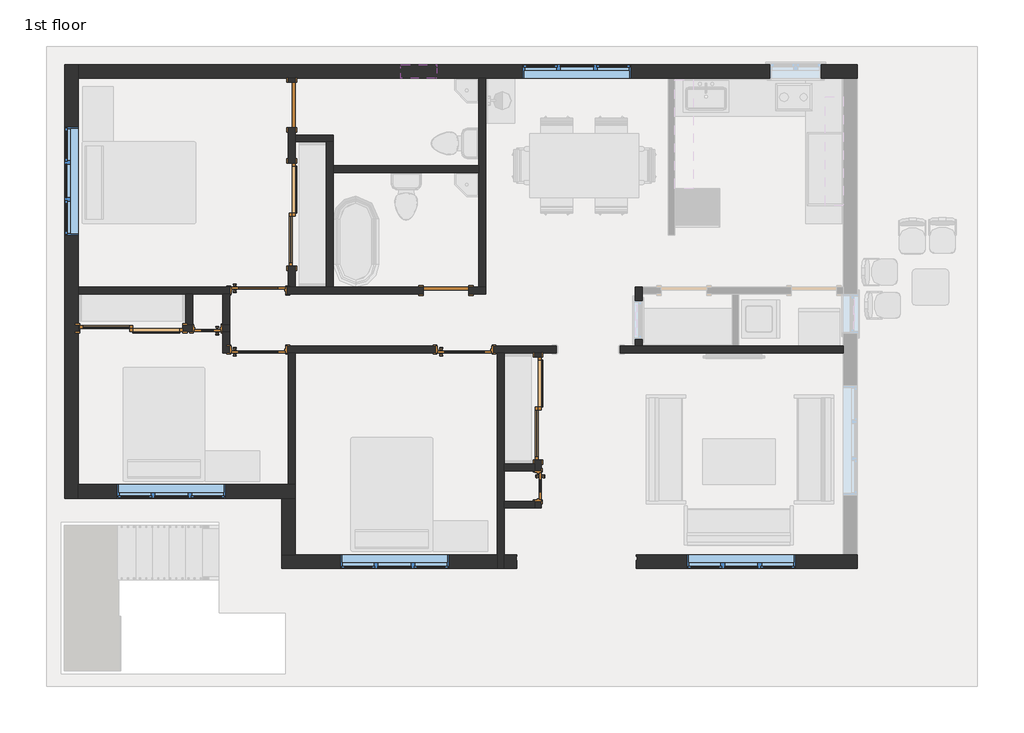
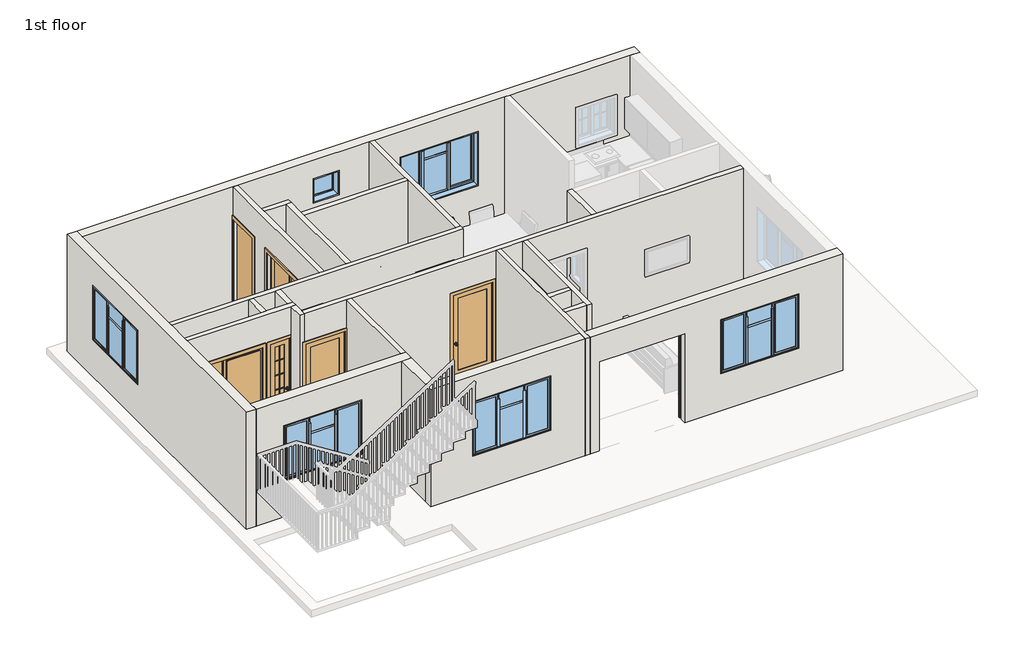
# One storey, part 1 of 4: 23 walls, 10 doors, 6 windows.
"""IFC4 building model written with IfcOpenShell, lengths in millimetres."""

from ifc_helpers import new_model, si_unit, frame, origin, place, context, project, spatial, polyline, outline, extrude, faceted_brep, transform, mapped, element, save
from components import door_505787c2, door_a3feeac7, door_3c6ab76a, door_ccf0cbd1, door_214872d5, door_78caadf7, window_80340324, window_7a1f68bc

model = new_model("IFC4")

# Units and contexts
model_context = context("Model", 3, world=origin())
ifc_project = project(units=[si_unit("LENGTHUNIT", "METRE", prefix="MILLI")], contexts=[model_context])

# Site, building, storey
site = spatial("IfcSite", under=ifc_project)
building = spatial("IfcBuilding", under=site)
storey = spatial("IfcBuildingStorey", under=building, Name="1st floor", Elevation=3810.0)

# Doors
placement = place(None, origin())
door_shape = door_505787c2(model_context)
element("IfcDoor", 1, ObjectType="Door-Double-Sliding : 68\" x 84\"", at=placement, inside=storey, context=model_context, shape_type="MappedRepresentation", body=[
    mapped(door_shape, transform((-1350.0263529, 910.5161978, 3810.0), x_axis=(0.0, -1.0, 0.0), y_axis=(1.0, 0.0, 0.0), z_axis=(0.0, 0.0, 1.0))),
])
element("IfcDoor", 2, ObjectType="Door-Double-Sliding : 68\" x 84\"", at=placement, inside=storey, context=model_context, shape_type="MappedRepresentation", body=[
    mapped(door_shape, transform((-8046.1013529, 2383.7161978, 3810.0), x_axis=(-1.0, 0.0, 0.0), y_axis=(0.0, -1.0, 0.0), z_axis=(0.0, 0.0, 1.0))),
])
element("IfcDoor", 3, ObjectType="Door-Double-Sliding : 68\" x 84\"", at=placement, inside=storey, context=model_context, shape_type="MappedRepresentation", body=[
    mapped(door_shape, transform((-5477.5263529, 4168.0661978, 3810.0), x_axis=(0.0, -1.0, 0.0), y_axis=(1.0, 0.0, 0.0), z_axis=(0.0, 0.0, 1.0))),
])
door_2_shape = door_a3feeac7(model_context)
element("IfcDoor", 4, ObjectType="Door-Interior-Single-1_Panel-Wood : 36\" x 84\"", at=placement, inside=storey, context=model_context, shape_type="MappedRepresentation", body=[
    mapped(door_2_shape, transform((-5912.5013529, 1897.9411978, 3810.0), x_axis=(1.0, 0.0, 0.0), y_axis=(0.0, 1.0, 0.0), z_axis=(0.0, 0.0, 1.0))),
])
element("IfcDoor", 5, ObjectType="Door-Interior-Single-1_Panel-Wood : 36\" x 84\"", at=placement, inside=storey, context=model_context, shape_type="MappedRepresentation", body=[
    mapped(door_2_shape, transform((-2454.9263529, 1897.9411978, 3810.0), x_axis=(1.0, 0.0, 0.0), y_axis=(0.0, 1.0, 0.0), z_axis=(0.0, 0.0, 1.0))),
])
door_3_shape = door_3c6ab76a(model_context)
element("IfcDoor", 6, ObjectType="Door-Interior-Single-1_Panel-Wood : 36\" x 84\"", at=placement, inside=storey, context=model_context, shape_type="MappedRepresentation", body=[
    mapped(door_3_shape, transform((-5912.5013529, 2894.8911978, 3810.0), x_axis=(1.0, 0.0, 0.0), y_axis=(0.0, 1.0, 0.0), z_axis=(0.0, 0.0, 1.0))),
])
door_4_shape = door_ccf0cbd1(model_context)
element("IfcDoor", 7, ObjectType="Door-Interior-Single-Full Glass-Wood : 18\" x 84\"", at=placement, inside=storey, context=model_context, shape_type="MappedRepresentation", body=[
    mapped(door_4_shape, transform((-1219.8513529, -391.2338022, 3810.0), x_axis=(0.0, -1.0, 0.0), y_axis=(1.0, 0.0, 0.0), z_axis=(0.0, 0.0, 1.0))),
])
element("IfcDoor", 8, ObjectType="Door-Interior-Single-Full Glass-Wood : 18\" x 84\"", at=placement, inside=storey, context=model_context, shape_type="MappedRepresentation", body=[
    mapped(door_4_shape, transform((-6766.5763529, 2253.5411978, 3810.0), x_axis=(-1.0, 0.0, 0.0), y_axis=(0.0, -1.0, 0.0), z_axis=(0.0, 0.0, 1.0))),
])
door_5_shape = door_214872d5(model_context)
element("IfcDoor", 9, ObjectType="Single-Flush : 30\" x 84\"", at=placement, inside=storey, context=model_context, shape_type="MappedRepresentation", body=[
    mapped(door_5_shape, transform((-2766.0763529, 2891.7161978, 3810.0), x_axis=(1.0, 0.0, 0.0), y_axis=(0.0, 1.0, 0.0), z_axis=(0.0, 0.0, 1.0))),
])
door_6_shape = door_78caadf7(model_context)
element("IfcDoor", 10, ObjectType="Single-Flush : 30\" x 84\"", at=placement, inside=storey, context=model_context, shape_type="MappedRepresentation", body=[
    mapped(door_6_shape, transform((-5350.5263529, 6006.3911978, 3810.0), x_axis=(0.0, 1.0, 0.0), y_axis=(-1.0, 0.0, 0.0), z_axis=(0.0, 0.0, 1.0))),
])

# Walls
element("IfcWall", 11, ObjectType="Generic - 4.5\"", at=placement, inside=storey, context=model_context, shape_type="Brep", body=[
    faceted_brep([(-5407.6763529, 6454.0661978, 3810.0), (-5407.6763529, 6387.3911978, 3810.0), (-5407.6763529, 6387.3911978, 5943.6), (-5407.6763529, 5625.3911978, 5943.6), (-5407.6763529, 5625.3911978, 3810.0), (-5407.6763529, 5031.6661978, 3810.0), (-5407.6763529, 5031.6661978, 5943.6), (-5407.6763529, 3304.4661978, 5943.6), (-5407.6763529, 3304.4661978, 3810.0), (-5407.6763529, 2948.8661978, 3810.0), (-5407.6763529, 2948.8661978, 6705.6), (-5407.6763529, 6454.0661978, 6705.6), (-5293.3763529, 6387.3911978, 5943.6), (-5293.3763529, 6387.3911978, 3810.0), (-5293.3763529, 6454.0661978, 3810.0), (-5293.3763529, 6454.0661978, 6705.6), (-5293.3763529, 5501.5661978, 6705.6), (-5293.3763529, 5387.2661978, 6705.6), (-5293.3763529, 2948.8661978, 6705.6), (-5293.3763529, 2948.8661978, 3810.0), (-5293.3763529, 3304.4661978, 3810.0), (-5293.3763529, 3304.4661978, 5943.6), (-5293.3763529, 5031.6661978, 5943.6), (-5293.3763529, 5031.6661978, 3810.0), (-5293.3763529, 5387.2661978, 3810.0), (-5293.3763529, 5501.5661978, 3810.0), (-5293.3763529, 5625.3911978, 3810.0), (-5293.3763529, 5625.3911978, 5943.6)], [[[0, 1, 2, 3, 4, 5, 6, 7, 8, 9, 10, 11]], [[12, 13, 14, 15, 16, 17, 18, 19, 20, 21, 22, 23, 24, 25, 26, 27]], [[9, 8, 20, 19]], [[14, 13, 1, 0]], [[26, 25, 24, 23, 5, 4]], [[11, 10, 18, 17, 16, 15]], [[0, 11, 15, 14]], [[10, 9, 19, 18]], [[23, 22, 6, 5]], [[21, 20, 8, 7]], [[22, 21, 7, 6]], [[2, 1, 13, 12]], [[3, 2, 12, 27]], [[4, 3, 27, 26]]]),
])
element("IfcWall", 12, ObjectType="Generic - 4.5\"", at=placement, inside=storey, context=model_context, shape_type="Brep", body=[
    faceted_brep([(-2099.3263529, 2948.8661978, 3810.0), (-2213.6263529, 2948.8661978, 3810.0), (-2385.0763529, 2948.8661978, 3810.0), (-2385.0763529, 2948.8661978, 5943.6), (-3147.0763529, 2948.8661978, 5943.6), (-3147.0763529, 2948.8661978, 3810.0), (-4658.3763529, 2948.8661978, 3810.0), (-4772.6763529, 2948.8661978, 3810.0), (-5293.3763529, 2948.8661978, 3810.0), (-5407.6763529, 2948.8661978, 3810.0), (-5429.9013529, 2948.8661978, 3810.0), (-5429.9013529, 2948.8661978, 5969.0), (-6395.1013529, 2948.8661978, 5969.0), (-6395.1013529, 2948.8661978, 3810.0), (-8931.9263529, 2948.8661978, 3810.0), (-8931.9263529, 2948.8661978, 6705.6), (-5407.6763529, 2948.8661978, 6705.6), (-5293.3763529, 2948.8661978, 6705.6), (-4772.6763529, 2948.8661978, 6705.6), (-4658.3763529, 2948.8661978, 6705.6), (-2213.6263529, 2948.8661978, 6705.6), (-2099.3263529, 2948.8661978, 6705.6), (-2385.0763529, 2834.5661978, 5943.6), (-2385.0763529, 2834.5661978, 3810.0), (-2099.3263529, 2834.5661978, 3810.0), (-2099.3263529, 2834.5661978, 6705.6), (-6391.9263529, 2834.5661978, 6705.6), (-6506.2263529, 2834.5661978, 6705.6), (-7014.2263529, 2834.5661978, 6705.6), (-7128.5263529, 2834.5661978, 6705.6), (-8931.9263529, 2834.5661978, 6705.6), (-8931.9263529, 2834.5661978, 3810.0), (-7128.5263529, 2834.5661978, 3810.0), (-7014.2263529, 2834.5661978, 3810.0), (-6506.2263529, 2834.5661978, 3810.0), (-6395.1013529, 2834.5661978, 3810.0), (-6395.1013529, 2834.5661978, 5969.0), (-5429.9013529, 2834.5661978, 5969.0), (-5429.9013529, 2834.5661978, 3810.0), (-3147.0763529, 2834.5661978, 3810.0), (-3147.0763529, 2834.5661978, 5943.6)], [[[0, 1, 2, 3, 4, 5, 6, 7, 8, 9, 10, 11, 12, 13, 14, 15, 16, 17, 18, 19, 20, 21]], [[22, 23, 24, 25, 26, 27, 28, 29, 30, 31, 32, 33, 34, 35, 36, 37, 38, 39, 40]], [[31, 14, 13, 35, 34, 33, 32]], [[39, 38, 10, 9, 8, 7, 6, 5]], [[24, 23, 2, 1, 0]], [[21, 20, 19, 18, 17, 16, 15, 30, 29, 28, 27, 26, 25]], [[15, 14, 31, 30]], [[0, 21, 25, 24]], [[37, 11, 10, 38]], [[11, 37, 36, 12]], [[12, 36, 35, 13]], [[3, 2, 23, 22]], [[4, 3, 22, 40]], [[5, 4, 40, 39]]]),
])
element("IfcWall", 13, ObjectType="Generic - 4.5\"", at=placement, inside=storey, context=model_context, shape_type="Brep", body=[
    faceted_brep([(-8931.9263529, 2199.5661978, 3810.0), (-8909.7013529, 2199.5661978, 3810.0), (-8909.7013529, 2199.5661978, 5943.6), (-7182.5013529, 2199.5661978, 5943.6), (-7182.5013529, 2199.5661978, 3810.0), (-7020.5763529, 2199.5661978, 3810.0), (-7020.5763529, 2199.5661978, 5969.0), (-6512.5763529, 2199.5661978, 5969.0), (-6512.5763529, 2199.5661978, 3810.0), (-6506.2263529, 2199.5661978, 3810.0), (-6391.9263529, 2199.5661978, 3810.0), (-6391.9263529, 2199.5661978, 6705.6), (-6506.2263529, 2199.5661978, 6705.6), (-8931.9263529, 2199.5661978, 6705.6), (-8909.7013529, 2313.8661978, 5943.6), (-8909.7013529, 2313.8661978, 3810.0), (-8931.9263529, 2313.8661978, 3810.0), (-8931.9263529, 2313.8661978, 6705.6), (-7128.5263529, 2313.8661978, 6705.6), (-7014.2263529, 2313.8661978, 6705.6), (-6506.2263529, 2313.8661978, 6705.6), (-6391.9263529, 2313.8661978, 6705.6), (-6391.9263529, 2313.8661978, 3810.0), (-6506.2263529, 2313.8661978, 3810.0), (-6512.5763529, 2313.8661978, 3810.0), (-6512.5763529, 2313.8661978, 5969.0), (-7020.5763529, 2313.8661978, 5969.0), (-7020.5763529, 2313.8661978, 3810.0), (-7128.5263529, 2313.8661978, 3810.0), (-7182.5013529, 2313.8661978, 3810.0), (-7182.5013529, 2313.8661978, 5943.6)], [[[0, 1, 2, 3, 4, 5, 6, 7, 8, 9, 10, 11, 12, 13]], [[14, 15, 16, 17, 18, 19, 20, 21, 22, 23, 24, 25, 26, 27, 28, 29, 30]], [[22, 10, 9, 8, 24, 23]], [[16, 15, 1, 0]], [[29, 28, 27, 5, 4]], [[13, 12, 11, 21, 20, 19, 18, 17]], [[0, 13, 17, 16]], [[11, 10, 22, 21]], [[26, 6, 5, 27]], [[6, 26, 25, 7]], [[7, 25, 24, 8]], [[4, 3, 30, 29]], [[2, 1, 15, 14]], [[3, 2, 14, 30]]]),
])
element("IfcWall", 14, ObjectType="Generic - 4.5\"", at=placement, inside=storey, context=model_context, shape_type="Brep", body=[
    faceted_brep([(-7014.2263529, 2313.8661978, 3810.0), (-7014.2263529, 2834.5661978, 3810.0), (-7014.2263529, 2834.5661978, 6705.6), (-7014.2263529, 2313.8661978, 6705.6), (-7128.5263529, 2313.8661978, 3810.0), (-7128.5263529, 2313.8661978, 6705.6), (-7128.5263529, 2834.5661978, 6705.6), (-7128.5263529, 2834.5661978, 3810.0), (-7020.5763529, 2313.8661978, 3810.0)], [[[0, 1, 2, 3]], [[4, 5, 6, 7]], [[1, 0, 8, 4, 7]], [[3, 2, 6, 5]], [[0, 3, 5, 4, 8]], [[2, 1, 7, 6]]]),
])
element("IfcWall", 15, ObjectType="Generic - 4.5\"", at=placement, inside=storey, context=model_context, shape_type="Brep", body=[
    faceted_brep([(-6391.9263529, 2313.8661978, 3810.0), (-6391.9263529, 2834.5661978, 3810.0), (-6391.9263529, 2834.5661978, 6705.6), (-6391.9263529, 2313.8661978, 6705.6), (-6506.2263529, 2313.8661978, 3810.0), (-6506.2263529, 2313.8661978, 6705.6), (-6506.2263529, 2834.5661978, 6705.6), (-6506.2263529, 2834.5661978, 3810.0), (-6395.1013529, 2834.5661978, 3810.0)], [[[0, 1, 2, 3]], [[4, 5, 6, 7]], [[1, 0, 4, 7, 8]], [[3, 2, 6, 5]], [[0, 3, 5, 4]], [[2, 1, 8, 7, 6]]]),
])
element("IfcWall", 16, ObjectType="Generic - 4.5\"", at=placement, inside=storey, context=model_context, shape_type="SweptSolid", body=[
    extrude(outline(polyline([(-5293.3763529, 1843.9661978), (-5293.3763529, -365.8338022), (-5407.6763529, -365.8338022), (-5407.6763529, 1843.9661978), (-5293.3763529, 1843.9661978)])), frame((0.0, 0.0, 3810.0), z_axis=(0.0, 0.0, 1.0), x_axis=(1.0, 0.0, 0.0)), (0.0, 0.0, 1.0), 2895.6),
])
element("IfcWall", 17, ObjectType="Generic - 4.5\"", at=placement, inside=storey, context=model_context, shape_type="Brep", body=[
    faceted_brep([(-6506.2263529, 2199.5661978, 3810.0), (-6506.2263529, 1843.9661978, 3810.0), (-6506.2263529, 1843.9661978, 6705.6), (-6506.2263529, 2199.5661978, 6705.6), (-6391.9263529, 2199.5661978, 6705.6), (-6391.9263529, 1958.2661978, 6705.6), (-6391.9263529, 1843.9661978, 6705.6), (-6391.9263529, 1843.9661978, 5969.0), (-6391.9263529, 1958.2661978, 5969.0), (-6391.9263529, 1958.2661978, 3810.0), (-6391.9263529, 2199.5661978, 3810.0), (-6395.1013529, 1958.2661978, 3810.0), (-6395.1013529, 1843.9661978, 3810.0), (-6395.1013529, 1843.9661978, 5969.0), (-6395.1013529, 1958.2661978, 5969.0)], [[[0, 1, 2, 3]], [[4, 5, 6, 7, 8, 9, 10]], [[1, 0, 10, 9, 11, 12]], [[3, 2, 6, 5, 4]], [[0, 3, 4, 10]], [[2, 1, 12, 13, 7, 6]], [[14, 11, 9, 8]], [[13, 14, 8, 7]], [[11, 14, 13, 12]]]),
])
element("IfcWall", 18, ObjectType="Generic - 4.5\"", at=placement, inside=storey, context=model_context, shape_type="Brep", body=[
    faceted_brep([(-1972.3263529, 1843.9661978, 3810.0), (-1902.4763529, 1843.9661978, 3810.0), (-1788.1763529, 1843.9661978, 3810.0), (-1280.1763529, 1843.9661978, 3810.0), (-1165.8763529, 1843.9661978, 3810.0), (-911.8763529, 1843.9661978, 3810.0), (-911.8763529, 1843.9661978, 5943.6), (154.9236471, 1843.9661978, 5943.6), (154.9236471, 1843.9661978, 3810.0), (3901.4236471, 1843.9661978, 3810.0), (3901.4236471, 1843.9661978, 6705.6), (-1165.8763529, 1843.9661978, 6705.6), (-1280.1763529, 1843.9661978, 6705.6), (-1788.1763529, 1843.9661978, 6705.6), (-1902.4763529, 1843.9661978, 6705.6), (-5293.3763529, 1843.9661978, 6705.6), (-5407.6763529, 1843.9661978, 6705.6), (-6391.9263529, 1843.9661978, 6705.6), (-6391.9263529, 1843.9661978, 5969.0), (-5429.9013529, 1843.9661978, 5969.0), (-5429.9013529, 1843.9661978, 3810.0), (-5407.6763529, 1843.9661978, 3810.0), (-5293.3763529, 1843.9661978, 3810.0), (-2937.5263529, 1843.9661978, 3810.0), (-2937.5263529, 1843.9661978, 5969.0), (-1972.3263529, 1843.9661978, 5969.0), (-911.8763529, 1958.2661978, 5943.6), (-911.8763529, 1958.2661978, 3810.0), (-1972.3263529, 1958.2661978, 3810.0), (-1972.3263529, 1958.2661978, 5969.0), (-2937.5263529, 1958.2661978, 5969.0), (-2937.5263529, 1958.2661978, 3810.0), (-5429.9013529, 1958.2661978, 3810.0), (-5429.9013529, 1958.2661978, 5969.0), (-6391.9263529, 1958.2661978, 5969.0), (-6391.9263529, 1958.2661978, 6705.6), (408.9236471, 1958.2661978, 6705.6), (523.2236471, 1958.2661978, 6705.6), (2034.5236471, 1958.2661978, 6705.6), (2148.8236471, 1958.2661978, 6705.6), (3901.4236471, 1958.2661978, 6705.6), (3901.4236471, 1958.2661978, 3810.0), (2148.8236471, 1958.2661978, 3810.0), (2034.5236471, 1958.2661978, 3810.0), (523.2236471, 1958.2661978, 3810.0), (408.9236471, 1958.2661978, 3810.0), (154.9236471, 1958.2661978, 3810.0), (154.9236471, 1958.2661978, 5943.6)], [[[0, 1, 2, 3, 4, 5, 6, 7, 8, 9, 10, 11, 12, 13, 14, 15, 16, 17, 18, 19, 20, 21, 22, 23, 24, 25]], [[26, 27, 28, 29, 30, 31, 32, 33, 34, 35, 36, 37, 38, 39, 40, 41, 42, 43, 44, 45, 46, 47]], [[20, 32, 31, 23, 22, 21]], [[28, 27, 5, 4, 3, 2, 1, 0]], [[46, 45, 44, 43, 42, 41, 9, 8]], [[17, 16, 15, 14, 13, 12, 11, 10, 40, 39, 38, 37, 36, 35]], [[17, 35, 34, 18]], [[10, 9, 41, 40]], [[19, 18, 34, 33]], [[25, 29, 28, 0]], [[29, 25, 24, 30]], [[30, 24, 23, 31]], [[19, 33, 32, 20]], [[8, 7, 47, 46]], [[6, 5, 27, 26]], [[7, 6, 26, 47]]]),
])
element("IfcWall", 19, ObjectType="Generic - 4.5\"", at=placement, inside=storey, context=model_context, shape_type="Brep", body=[
    faceted_brep([(-1902.4763529, 1843.9661978, 3810.0), (-1902.4763529, -1546.9338022, 3810.0), (-1902.4763529, -1775.5338022, 3810.0), (-1902.4763529, -1775.5338022, 6705.6), (-1902.4763529, -1546.9338022, 6705.6), (-1902.4763529, 1843.9661978, 6705.6), (-1788.1763529, 1843.9661978, 3810.0), (-1788.1763529, 1843.9661978, 6705.6), (-1788.1763529, -22.9338022, 6705.6), (-1788.1763529, -137.2338022, 6705.6), (-1788.1763529, -645.2338022, 6705.6), (-1788.1763529, -759.5338022, 6705.6), (-1788.1763529, -1546.9338022, 6705.6), (-1788.1763529, -1775.5338022, 6705.6), (-1788.1763529, -1775.5338022, 3810.0), (-1788.1763529, -1546.9338022, 3810.0), (-1788.1763529, -759.5338022, 3810.0), (-1788.1763529, -645.2338022, 3810.0), (-1788.1763529, -137.2338022, 3810.0), (-1788.1763529, -22.9338022, 3810.0)], [[[0, 1, 2, 3, 4, 5]], [[6, 7, 8, 9, 10, 11, 12, 13, 14, 15, 16, 17, 18, 19]], [[2, 1, 0, 6, 19, 18, 17, 16, 15, 14]], [[5, 4, 3, 13, 12, 11, 10, 9, 8, 7]], [[0, 5, 7, 6]], [[3, 2, 14, 13]]]),
])
element("IfcWall", 20, ObjectType="Generic - 4.5\"", at=placement, inside=storey, context=model_context, shape_type="Brep", body=[
    faceted_brep([(-1280.1763529, 46.9161978, 5943.6), (-1280.1763529, 46.9161978, 3810.0), (-1280.1763529, -22.9338022, 3810.0), (-1280.1763529, -137.2338022, 3810.0), (-1280.1763529, -137.2338022, 5969.0), (-1280.1763529, -645.2338022, 5969.0), (-1280.1763529, -645.2338022, 3810.0), (-1280.1763529, -759.5338022, 3810.0), (-1280.1763529, -759.5338022, 6705.6), (-1280.1763529, -645.2338022, 6705.6), (-1280.1763529, -137.2338022, 6705.6), (-1280.1763529, -22.9338022, 6705.6), (-1280.1763529, 1843.9661978, 6705.6), (-1280.1763529, 1843.9661978, 3810.0), (-1280.1763529, 1774.1161978, 3810.0), (-1280.1763529, 1774.1161978, 5943.6), (-1165.8763529, -137.2338022, 3810.0), (-1165.8763529, 46.9161978, 3810.0), (-1165.8763529, 46.9161978, 5943.6), (-1165.8763529, 1774.1161978, 5943.6), (-1165.8763529, 1774.1161978, 3810.0), (-1165.8763529, 1843.9661978, 3810.0), (-1165.8763529, 1843.9661978, 6705.6), (-1165.8763529, -759.5338022, 6705.6), (-1165.8763529, -759.5338022, 3810.0), (-1165.8763529, -645.2338022, 3810.0), (-1165.8763529, -645.2338022, 5969.0), (-1165.8763529, -137.2338022, 5969.0)], [[[0, 1, 2, 3, 4, 5, 6, 7, 8, 9, 10, 11, 12, 13, 14, 15]], [[16, 17, 18, 19, 20, 21, 22, 23, 24, 25, 26, 27]], [[24, 7, 6, 25]], [[14, 13, 21, 20]], [[3, 2, 1, 17, 16]], [[12, 11, 10, 9, 8, 23, 22]], [[13, 12, 22, 21]], [[8, 7, 24, 23]], [[5, 26, 25, 6]], [[26, 5, 4, 27]], [[27, 4, 3, 16]], [[20, 19, 15, 14]], [[18, 17, 1, 0]], [[19, 18, 0, 15]]]),
])
element("IfcWall", 21, ObjectType="Generic - 4.5\"", at=placement, inside=storey, context=model_context, shape_type="Brep", body=[
    faceted_brep([(-1280.1763529, -22.9338022, 3810.0), (-1788.1763529, -22.9338022, 3810.0), (-1788.1763529, -22.9338022, 6705.6), (-1280.1763529, -22.9338022, 6705.6), (-1280.1763529, -137.2338022, 3810.0), (-1280.1763529, -137.2338022, 5969.0), (-1280.1763529, -137.2338022, 6705.6), (-1788.1763529, -137.2338022, 6705.6), (-1788.1763529, -137.2338022, 3810.0)], [[[0, 1, 2, 3]], [[4, 5, 6, 7, 8]], [[1, 0, 4, 8]], [[3, 2, 7, 6]], [[0, 3, 6, 5, 4]], [[2, 1, 8, 7]]]),
])
element("IfcWall", 22, ObjectType="Generic - 4.5\"", at=placement, inside=storey, context=model_context, shape_type="Brep", body=[
    faceted_brep([(-1280.1763529, -645.2338022, 3810.0), (-1788.1763529, -645.2338022, 3810.0), (-1788.1763529, -645.2338022, 6705.6), (-1280.1763529, -645.2338022, 6705.6), (-1280.1763529, -645.2338022, 5969.0), (-1280.1763529, -759.5338022, 3810.0), (-1280.1763529, -759.5338022, 6705.6), (-1788.1763529, -759.5338022, 6705.6), (-1788.1763529, -759.5338022, 3810.0)], [[[0, 1, 2, 3, 4]], [[5, 6, 7, 8]], [[1, 0, 5, 8]], [[3, 2, 7, 6]], [[0, 4, 3, 6, 5]], [[2, 1, 8, 7]]]),
])
element("IfcWall", 23, ObjectType="Generic - 4.5\"", at=placement, inside=storey, context=model_context, shape_type="Brep", body=[
    faceted_brep([(-2099.3263529, 2948.8661978, 3810.0), (-2099.3263529, 6454.0661978, 3810.0), (-2099.3263529, 6454.0661978, 6705.6), (-2099.3263529, 2948.8661978, 6705.6), (-2213.6263529, 2948.8661978, 3810.0), (-2213.6263529, 2948.8661978, 6705.6), (-2213.6263529, 4872.9161978, 6705.6), (-2213.6263529, 4987.2161978, 6705.6), (-2213.6263529, 6454.0661978, 6705.6), (-2213.6263529, 6454.0661978, 3810.0), (-2213.6263529, 4987.2161978, 3810.0), (-2213.6263529, 4872.9161978, 3810.0)], [[[0, 1, 2, 3]], [[4, 5, 6, 7, 8, 9, 10, 11]], [[1, 0, 4, 11, 10, 9]], [[3, 2, 8, 7, 6, 5]], [[2, 1, 9, 8]], [[0, 3, 5, 4]]]),
])
element("IfcWall", 24, ObjectType="Generic - 4.5\"", at=placement, inside=storey, context=model_context, shape_type="Brep", body=[
    faceted_brep([(-5293.3763529, 5387.2661978, 3810.0), (-4772.6763529, 5387.2661978, 3810.0), (-4658.3763529, 5387.2661978, 3810.0), (-4658.3763529, 5387.2661978, 6705.6), (-4772.6763529, 5387.2661978, 6705.6), (-5293.3763529, 5387.2661978, 6705.6), (-5293.3763529, 5501.5661978, 3810.0), (-5293.3763529, 5501.5661978, 6705.6), (-4658.3763529, 5501.5661978, 6705.6), (-4658.3763529, 5501.5661978, 3810.0)], [[[0, 1, 2, 3, 4, 5]], [[6, 7, 8, 9]], [[2, 1, 0, 6, 9]], [[5, 4, 3, 8, 7]], [[0, 5, 7, 6]], [[3, 2, 9, 8]]]),
])
element("IfcWall", 25, ObjectType="Generic - 4.5\"", at=placement, inside=storey, context=model_context, shape_type="Brep", body=[
    faceted_brep([(-4772.6763529, 5387.2661978, 3810.0), (-4772.6763529, 2948.8661978, 3810.0), (-4772.6763529, 2948.8661978, 6705.6), (-4772.6763529, 5387.2661978, 6705.6), (-4658.3763529, 5387.2661978, 3810.0), (-4658.3763529, 5387.2661978, 6705.6), (-4658.3763529, 4987.2161978, 6705.6), (-4658.3763529, 4872.9161978, 6705.6), (-4658.3763529, 2948.8661978, 6705.6), (-4658.3763529, 2948.8661978, 3810.0), (-4658.3763529, 4872.9161978, 3810.0), (-4658.3763529, 4987.2161978, 3810.0)], [[[0, 1, 2, 3]], [[4, 5, 6, 7, 8, 9, 10, 11]], [[1, 0, 4, 11, 10, 9]], [[3, 2, 8, 7, 6, 5]], [[0, 3, 5, 4]], [[2, 1, 9, 8]]]),
])
element("IfcWall", 26, ObjectType="Generic - 4.5\"", at=placement, inside=storey, context=model_context, shape_type="SweptSolid", body=[
    extrude(outline(polyline([(-4658.3763529, 4987.2161978), (-2213.6263529, 4987.2161978), (-2213.6263529, 4872.9161978), (-4658.3763529, 4872.9161978), (-4658.3763529, 4987.2161978)])), frame((0.0, 0.0, 3810.0), z_axis=(0.0, 0.0, 1.0), x_axis=(1.0, 0.0, 0.0)), (0.0, 0.0, 1.0), 2895.6),
])
element("IfcWall", 27, ObjectType="Generic - 4.5\"", at=placement, inside=storey, context=model_context, shape_type="Brep", body=[
    faceted_brep([(523.2236471, 1958.2661978, 3810.0), (523.2236471, 2834.5661978, 3810.0), (523.2236471, 2948.8661978, 3810.0), (523.2236471, 2948.8661978, 6705.6), (523.2236471, 2834.5661978, 6705.6), (523.2236471, 1958.2661978, 6705.6), (523.2236471, 2726.6161978, 5791.2), (523.2236471, 2726.6161978, 4724.4), (523.2236471, 2066.2161978, 4724.4), (523.2236471, 2066.2161978, 5791.2), (408.9236471, 1958.2661978, 3810.0), (408.9236471, 1958.2661978, 6705.6), (408.9236471, 2948.8661978, 6705.6), (408.9236471, 2948.8661978, 3810.0), (408.9236471, 2726.6161978, 5791.2), (408.9236471, 2066.2161978, 5791.2), (408.9236471, 2066.2161978, 4724.4), (408.9236471, 2726.6161978, 4724.4)], [[[0, 1, 2, 3, 4, 5], [6, 7, 8, 9]], [[10, 11, 12, 13], [14, 15, 16, 17]], [[2, 1, 0, 10, 13]], [[5, 4, 3, 12, 11]], [[0, 5, 11, 10]], [[3, 2, 13, 12]], [[7, 6, 14, 17]], [[8, 7, 17, 16]], [[9, 8, 16, 15]], [[6, 9, 15, 14]]]),
])
element("IfcWall", 28, ObjectType="Generic - 9\"", at=placement, inside=storey, context=model_context, shape_type="Brep", body=[
    faceted_brep([(-9160.5263529, 6682.6661978, 3810.0), (-9160.5263529, -594.4338022, 3810.0), (-9160.5263529, -594.4338022, 6705.6), (-9160.5263529, 6682.6661978, 6705.6), (-9160.5263529, 5644.4411978, 6070.6), (-9160.5263529, 3815.6411978, 6070.6), (-9160.5263529, 3815.6411978, 4724.4), (-9160.5263529, 5644.4411978, 4724.4), (-8931.9263529, 6682.6661978, 3810.0), (-8931.9263529, 6682.6661978, 6705.6), (-8931.9263529, 6454.0661978, 6705.6), (-8931.9263529, 2948.8661978, 6705.6), (-8931.9263529, 2834.5661978, 6705.6), (-8931.9263529, 2313.8661978, 6705.6), (-8931.9263529, 2199.5661978, 6705.6), (-8931.9263529, -365.8338022, 6705.6), (-8931.9263529, -594.4338022, 6705.6), (-8931.9263529, -594.4338022, 3810.0), (-8931.9263529, -365.8338022, 3810.0), (-8931.9263529, 2199.5661978, 3810.0), (-8931.9263529, 2313.8661978, 3810.0), (-8931.9263529, 2834.5661978, 3810.0), (-8931.9263529, 2948.8661978, 3810.0), (-8931.9263529, 6454.0661978, 3810.0), (-8931.9263529, 5644.4411978, 6070.6), (-8931.9263529, 5644.4411978, 4724.4), (-8931.9263529, 3815.6411978, 4724.4), (-8931.9263529, 3815.6411978, 6070.6)], [[[0, 1, 2, 3], [4, 5, 6, 7]], [[8, 9, 10, 11, 12, 13, 14, 15, 16, 17, 18, 19, 20, 21, 22, 23], [24, 25, 26, 27]], [[1, 0, 8, 23, 22, 21, 20, 19, 18, 17]], [[3, 2, 16, 15, 14, 13, 12, 11, 10, 9]], [[0, 3, 9, 8]], [[2, 1, 17, 16]], [[25, 24, 4, 7]], [[26, 25, 7, 6]], [[27, 26, 6, 5]], [[24, 27, 5, 4]]]),
])
element("IfcWall", 29, ObjectType="Generic - 9\"", at=placement, inside=storey, context=model_context, shape_type="Brep", body=[
    faceted_brep([(-8931.9263529, 6454.0661978, 3810.0), (-5407.6763529, 6454.0661978, 3810.0), (-5293.3763529, 6454.0661978, 3810.0), (-2213.6263529, 6454.0661978, 3810.0), (-2099.3263529, 6454.0661978, 3810.0), (961.3736471, 6454.0661978, 3810.0), (1075.6736471, 6454.0661978, 3810.0), (3901.4236471, 6454.0661978, 3810.0), (4130.0236471, 6454.0661978, 3810.0), (4130.0236471, 6454.0661978, 6705.6), (3901.4236471, 6454.0661978, 6705.6), (1075.6736471, 6454.0661978, 6705.6), (961.3736471, 6454.0661978, 6705.6), (-2099.3263529, 6454.0661978, 6705.6), (-2213.6263529, 6454.0661978, 6705.6), (-5293.3763529, 6454.0661978, 6705.6), (-5407.6763529, 6454.0661978, 6705.6), (-8931.9263529, 6454.0661978, 6705.6), (3533.1236471, 6454.0661978, 5816.6), (3533.1236471, 6454.0661978, 4902.2), (2669.5236471, 6454.0661978, 4902.2), (2669.5236471, 6454.0661978, 5816.6), (345.4236471, 6454.0661978, 6070.6), (345.4236471, 6454.0661978, 4724.4), (-1483.3763529, 6454.0661978, 4724.4), (-1483.3763529, 6454.0661978, 6070.6), (-2918.4763529, 6454.0661978, 6248.4), (-2918.4763529, 6454.0661978, 5638.8), (-3528.0763529, 6454.0661978, 5638.8), (-3528.0763529, 6454.0661978, 6248.4), (-8931.9263529, 6682.6661978, 3810.0), (-8931.9263529, 6682.6661978, 6705.6), (4130.0236471, 6682.6661978, 6705.6), (4130.0236471, 6682.6661978, 3810.0), (3533.1236471, 6682.6661978, 5816.6), (2669.5236471, 6682.6661978, 5816.6), (2669.5236471, 6682.6661978, 4902.2), (3533.1236471, 6682.6661978, 4902.2), (345.4236471, 6682.6661978, 6070.6), (-1483.3763529, 6682.6661978, 6070.6), (-1483.3763529, 6682.6661978, 4724.4), (345.4236471, 6682.6661978, 4724.4), (-2918.4763529, 6682.6661978, 6248.4), (-3528.0763529, 6682.6661978, 6248.4), (-3528.0763529, 6682.6661978, 5638.8), (-2918.4763529, 6682.6661978, 5638.8)], [[[0, 1, 2, 3, 4, 5, 6, 7, 8, 9, 10, 11, 12, 13, 14, 15, 16, 17], [18, 19, 20, 21], [22, 23, 24, 25], [26, 27, 28, 29]], [[30, 31, 32, 33], [34, 35, 36, 37], [38, 39, 40, 41], [42, 43, 44, 45]], [[8, 7, 6, 5, 4, 3, 2, 1, 0, 30, 33]], [[17, 16, 15, 14, 13, 12, 11, 10, 9, 32, 31]], [[0, 17, 31, 30]], [[9, 8, 33, 32]], [[19, 18, 34, 37]], [[20, 19, 37, 36]], [[21, 20, 36, 35]], [[18, 21, 35, 34]], [[23, 22, 38, 41]], [[24, 23, 41, 40]], [[25, 24, 40, 39]], [[22, 25, 39, 38]], [[27, 26, 42, 45]], [[28, 27, 45, 44]], [[29, 28, 44, 43]], [[26, 29, 43, 42]]]),
])
element("IfcWall", 30, ObjectType="Generic - 9\"", at=placement, inside=storey, context=model_context, shape_type="Brep", body=[
    faceted_brep([(-8931.9263529, -594.4338022, 3810.0), (-5521.9763529, -594.4338022, 3810.0), (-5293.3763529, -594.4338022, 3810.0), (-5293.3763529, -594.4338022, 6705.6), (-5521.9763529, -594.4338022, 6705.6), (-8931.9263529, -594.4338022, 6705.6), (-8284.2263529, -594.4338022, 6070.6), (-6455.4263529, -594.4338022, 6070.6), (-6455.4263529, -594.4338022, 4724.4), (-8284.2263529, -594.4338022, 4724.4), (-8931.9263529, -365.8338022, 3810.0), (-8931.9263529, -365.8338022, 6705.6), (-5407.6763529, -365.8338022, 6705.6), (-5293.3763529, -365.8338022, 6705.6), (-5293.3763529, -365.8338022, 3810.0), (-5407.6763529, -365.8338022, 3810.0), (-8284.2263529, -365.8338022, 6070.6), (-8284.2263529, -365.8338022, 4724.4), (-6455.4263529, -365.8338022, 4724.4), (-6455.4263529, -365.8338022, 6070.6)], [[[0, 1, 2, 3, 4, 5], [6, 7, 8, 9]], [[10, 11, 12, 13, 14, 15], [16, 17, 18, 19]], [[2, 1, 0, 10, 15, 14]], [[5, 4, 3, 13, 12, 11]], [[3, 2, 14, 13]], [[0, 5, 11, 10]], [[17, 16, 6, 9]], [[18, 17, 9, 8]], [[19, 18, 8, 7]], [[16, 19, 7, 6]]]),
])
element("IfcWall", 31, ObjectType="Generic - 9\"", at=placement, inside=storey, context=model_context, shape_type="Brep", body=[
    faceted_brep([(-1902.4763529, -1546.9338022, 3810.0), (-5293.3763529, -1546.9338022, 3810.0), (-5521.9763529, -1546.9338022, 3810.0), (-5521.9763529, -1546.9338022, 6705.6), (-5293.3763529, -1546.9338022, 6705.6), (-1902.4763529, -1546.9338022, 6705.6), (-4540.9013529, -1546.9338022, 6070.6), (-4540.9013529, -1546.9338022, 4724.4), (-2712.1013529, -1546.9338022, 4724.4), (-2712.1013529, -1546.9338022, 6070.6), (-1902.4763529, -1775.5338022, 3810.0), (-1902.4763529, -1775.5338022, 6705.6), (-5521.9763529, -1775.5338022, 6705.6), (-5521.9763529, -1775.5338022, 3810.0), (-4540.9013529, -1775.5338022, 6070.6), (-2712.1013529, -1775.5338022, 6070.6), (-2712.1013529, -1775.5338022, 4724.4), (-4540.9013529, -1775.5338022, 4724.4)], [[[0, 1, 2, 3, 4, 5], [6, 7, 8, 9]], [[10, 11, 12, 13], [14, 15, 16, 17]], [[2, 1, 0, 10, 13]], [[5, 4, 3, 12, 11]], [[0, 5, 11, 10]], [[3, 2, 13, 12]], [[7, 6, 14, 17]], [[8, 7, 17, 16]], [[9, 8, 16, 15]], [[6, 9, 15, 14]]]),
])
element("IfcWall", 32, ObjectType="Generic - 9\"", at=placement, inside=storey, context=model_context, shape_type="SweptSolid", body=[
    extrude(outline(polyline([(-5521.9763529, -1546.9338022), (-5521.9763529, -594.4338022), (-5293.3763529, -594.4338022), (-5293.3763529, -1546.9338022), (-5521.9763529, -1546.9338022)])), frame((0.0, 0.0, 3810.0), z_axis=(0.0, 0.0, 1.0), x_axis=(1.0, 0.0, 0.0)), (0.0, 0.0, 1.0), 2895.6),
])
element("IfcWall", 33, ObjectType="Generic - 9\"", at=placement, inside=storey, context=model_context, shape_type="Brep", body=[
    faceted_brep([(4130.0236471, -1775.5338022, 6705.6), (-1788.1763529, -1775.5338022, 6705.6), (-1788.1763529, -1775.5338022, 3810.0), (-1575.3263529, -1775.5338022, 3810.0), (-1575.3263529, -1775.5338022, 6019.0), (424.6736471, -1775.5338022, 6019.0), (424.6736471, -1775.5338022, 3810.0), (4130.0236471, -1775.5338022, 3810.0), (1272.5236471, -1775.5338022, 6070.6), (3101.3236471, -1775.5338022, 6070.6), (3101.3236471, -1775.5338022, 4724.4), (1272.5236471, -1775.5338022, 4724.4), (-1788.1763529, -1546.9338022, 6705.6), (3901.4236471, -1546.9338022, 6705.6), (4130.0236471, -1546.9338022, 6705.6), (4130.0236471, -1546.9338022, 3810.0), (3901.4236471, -1546.9338022, 3810.0), (424.6736471, -1546.9338022, 3810.0), (424.6736471, -1546.9338022, 6019.0), (-1575.3263529, -1546.9338022, 6019.0), (-1575.3263529, -1546.9338022, 3810.0), (-1788.1763529, -1546.9338022, 3810.0), (1272.5236471, -1546.9338022, 6070.6), (1272.5236471, -1546.9338022, 4724.4), (3101.3236471, -1546.9338022, 4724.4), (3101.3236471, -1546.9338022, 6070.6), (-1575.3263529, -1566.9338022, 3810.0), (-1590.3263529, -1566.9338022, 3810.0), (-1590.3263529, -1636.9338022, 3810.0), (-1575.3263529, -1636.9338022, 3810.0), (424.6736471, -1636.9338022, 3810.0), (439.6736471, -1636.9338022, 3810.0), (439.6736471, -1566.9338022, 3810.0), (424.6736471, -1566.9338022, 3810.0), (424.6736471, -1566.9338022, 6019.0), (-1575.3263529, -1566.9338022, 6019.0), (-1575.3263529, -1636.9338022, 6019.0), (424.6736471, -1636.9338022, 6019.0), (-1590.3263529, -1636.9338022, 6034.0), (439.6736471, -1636.9338022, 6034.0), (439.6736471, -1566.9338022, 6034.0), (-1590.3263529, -1566.9338022, 6034.0)], [[[0, 1, 2, 3, 4, 5, 6, 7], [8, 9, 10, 11]], [[12, 13, 14, 15, 16, 17, 18, 19, 20, 21], [22, 23, 24, 25]], [[2, 21, 20, 26, 27, 28, 29, 3]], [[15, 7, 6, 30, 31, 32, 33, 17, 16]], [[1, 0, 14, 13, 12]], [[2, 1, 12, 21]], [[0, 7, 15, 14]], [[34, 35, 19, 18]], [[36, 37, 5, 4]], [[29, 36, 4, 3]], [[37, 30, 6, 5]], [[37, 36, 29, 28, 38, 39, 31, 30]], [[31, 39, 40, 32]], [[35, 34, 33, 32, 40, 41, 27, 26]], [[33, 34, 18, 17]], [[35, 26, 20, 19]], [[38, 28, 27, 41]], [[39, 38, 41, 40]], [[23, 22, 8, 11]], [[24, 23, 11, 10]], [[25, 24, 10, 9]], [[22, 25, 9, 8]]]),
])

# Windows
window_shape = window_80340324(model_context)
element("IfcWindow", 34, ObjectType="Fixed : 24\" x 24\"", at=placement, inside=storey, context=model_context, shape_type="MappedRepresentation", body=[
    mapped(window_shape, transform((-3185.1763529, 6568.3661978, 4724.4), x_axis=(1.0, 0.0, 0.0), y_axis=(0.0, 1.0, 0.0), z_axis=(0.0, 0.0, 1.0))),
])
window_2_shape = window_7a1f68bc(model_context)
element("IfcWindow", 35, ObjectType="Window-Casement-Triple-Middle-Transom : 72\" x 53\"", at=placement, inside=storey, context=model_context, shape_type="MappedRepresentation", body=[
    mapped(window_2_shape, transform((-3626.5013529, -1661.2338022, 3810.0), x_axis=(-1.0, 0.0, 0.0), y_axis=(0.0, -1.0, 0.0), z_axis=(0.0, 0.0, 1.0))),
])
element("IfcWindow", 36, ObjectType="Window-Casement-Triple-Middle-Transom : 72\" x 53\"", at=placement, inside=storey, context=model_context, shape_type="MappedRepresentation", body=[
    mapped(window_2_shape, transform((-7369.8263529, -480.1338022, 3810.0), x_axis=(-1.0, 0.0, 0.0), y_axis=(0.0, -1.0, 0.0), z_axis=(0.0, 0.0, 1.0))),
])
element("IfcWindow", 37, ObjectType="Window-Casement-Triple-Middle-Transom : 72\" x 53\"", at=placement, inside=storey, context=model_context, shape_type="MappedRepresentation", body=[
    mapped(window_2_shape, transform((-9046.2263529, 4730.0411978, 3810.0), x_axis=(0.0, 1.0, 0.0), y_axis=(-1.0, 0.0, 0.0), z_axis=(0.0, 0.0, 1.0))),
])
element("IfcWindow", 38, ObjectType="Window-Casement-Triple-Middle-Transom : 72\" x 53\"", at=placement, inside=storey, context=model_context, shape_type="MappedRepresentation", body=[
    mapped(window_2_shape, transform((-568.9763529, 6568.3661978, 3810.0), x_axis=(1.0, 0.0, 0.0), y_axis=(0.0, 1.0, 0.0), z_axis=(0.0, 0.0, 1.0))),
])
element("IfcWindow", 39, ObjectType="Window-Casement-Triple-Middle-Transom : 72\" x 53\"", at=placement, inside=storey, context=model_context, shape_type="MappedRepresentation", body=[
    mapped(window_2_shape, transform((2186.9236471, -1661.2338022, 3810.0), x_axis=(-1.0, 0.0, 0.0), y_axis=(0.0, -1.0, 0.0), z_axis=(0.0, 0.0, 1.0))),
])

save(model, "model.ifc")

# Revit data of these elements
# Type "Door-Double-Sliding : 68\" x 84\""
#   Type Mark = "14"
#   Construction Type Id = "opn-d45"
#   Assembly Code = "C1020"
#   Analytic Construction = "Wood frame, double glass door "
#   Thickness = 0' - 2"
#   Thermal Resistance (R) = 1.8150 (h·ft²·°F)/BTU
#   Heat Transfer Coefficient (U) = 0.5510 BTU/(h·ft²·°F)
#   Height = 7' - 0"
#   Rail Width = 0' - 2"
#   Stiles = 0' - 2"
#   Trim Projection Ext = 0' - 1"
#   Trim Projection Int = 0' - 1"
#   Trim Width = 0' - 3"
#   Width = 5' - 8"
#   Define Thermal Properties by = 1
#   Glazing = Glass
#   Panel Material = Wood - Birch - Solid Stained Light Low Gloss
#   Trim Material = Paint - Sienna
#   Visual Light Transmittance = 0
#   Solar Heat Gain Coefficient = 0
#   Function = (empty or 0)
#   Wall Closure = (empty or 0)
# Type "Door-Interior-Single-1_Panel-Wood : 36\" x 84\""
#   Type Mark = "15"
#   Assembly Code = "C1020300"
#   Analytic Construction = "Wooden"
#   Top Rail = 0' - 4 11/16"
#   Thickness = 0' - 1 3/8"
#   Thermal Resistance (R) = 2.5876 (h·ft²·°F)/BTU
#   Swing Angle [instance default] = 90.00°
#   Stiles = 0' - 4 3/4"
#   Rough Width = 3' - 2"
#   Rough Height = 7' - 1"
#   Height = 7' - 0"
#   Width = 3' - 0"
#   Heat Transfer Coefficient (U) = 0.3865 BTU/(h·ft²·°F)
#   Bottom Rail = 0' - 9 1/8"
#   Trim Material = Cherry
#   Panel Material = Cherry
#   Frame Material = Cherry
#   Door Handle Material = Aluminum
#   Visual Light Transmittance = 0
#   Solar Heat Gain Coefficient = 0
#   Wall Closure = (empty or 0)
#   Function = (empty or 0)
# Type "Door-Interior-Single-Full Glass-Wood : 18\" x 84\""
#   Type Mark = "13"
#   Assembly Code = "C1020300"
#   Analytic Construction = "Wood frame with single clear glass"
#   Top Rail = 0' - 4 11/16"
#   Thickness = 0' - 1 3/8"
#   Thermal Resistance (R) = 1.0102 (h·ft²·°F)/BTU
#   Swing Angle [instance default] = 90.00°
#   Stiles = 0' - 4 3/4"
#   Rough Width = 1' - 8"
#   Rough Height = 7' - 1"
#   Height = 7' - 0"
#   Width = 1' - 6"
#   Heat Transfer Coefficient (U) = 0.9900 BTU/(h·ft²·°F)
#   Bottom Rail = 0' - 9 1/8"
#   Show Grill [instance default] = yes
#   Trim Material = Cherry
#   Panel Material = Cherry
#   Frame Material = Cherry
#   Door Handle Material = Aluminum
#   Visual Light Transmittance = 0
#   Solar Heat Gain Coefficient = 0
#   Wall Closure = (empty or 0)
#   Function = (empty or 0)
# Type "Single-Flush : 30\" x 84\""
#   Type Mark = "4"
#   Construction Type Id = "MDOOR"
#   Assembly Code = "C1020"
#   Analytic Construction = "Metal"
#   Thickness = 0' - 2"
#   Heat Transfer Coefficient (U) = 0.651978 BTU/(h·ft²·°F)
#   Height = 7' - 0"
#   Trim Projection Ext = 0' - 1"
#   Trim Projection Int = 0' - 1"
#   Trim Width = 0' - 3"
#   Width = 2' - 6"
#   Define Thermal Properties by = 1
#   Define Thermal Properties by = 1
#   Door Material = Door - Panel
#   Frame Material = Door - Frame
#   Visual Light Transmittance = 0
#   Solar Heat Gain Coefficient = 0
#   Function = (empty or 0)
#   Wall Closure = (empty or 0)
# Type "Generic - 4.5\""
#   Assembly Code = "B2010"
#   Layers, outside or top first: 0' - 4 1/2" no material (function 1)
# Type "Generic - 9\""
#   Assembly Code = "B2010"
#   Layers, outside or top first: 0' - 9" no material (function 1)
# Type "Fixed : 24\" x 24\""
#   Type Mark = "3"
#   Construction Type Id = "GSP4R"
#   Assembly Code = "B2020100"
#   Analytic Construction = "1/8 in Pilkington single glazing"
#   Visual Light Transmittance = 0.9
#   Solar Heat Gain Coefficient = 0.78
#   Heat Transfer Coefficient (U) = 0.6496 BTU/(h·ft²·°F)
#   Height = 2' - 0"
#   Default Sill Height = 3' - 0"
#   Width = 2' - 0"
#   Window Inset = 0' - 0 3/4"
#   Define Thermal Properties by = 1
#   Define Thermal Properties by = 1
#   Glass Pane Material = Glass
#   Sash Material = Sash
#   Wall Closure = (empty or 0)
# Type "Window-Casement-Triple-Middle-Transom : 72\" x 53\""
#   Type Mark = "18"
#   Fire Rating = "0.5h"
#   Assembly Code = "B2020100"
#   Analytic Construction = "Double glazing - domestic"
#   Window Width = 2' - 0"
#   Window Inset [instance default] = 0' - 0 5/8"
#   Wall Thickness [instance default] = 0' - 6"
#   Visual Light Transmittance = 0.81
#   Transom Height Ratio = 0.3
#   Thermal Resistance (R) = 1.8146 (h·ft²·°F)/BTU
#   Solar Heat Gain Coefficient = 0.76
#   Rough Width = 6' - 0 1/2"
#   Rough Height = 4' - 5 1/2"
#   Heat Transfer Coefficient (U) = 0.5511 BTU/(h·ft²·°F)
#   Height = 4' - 5"
#   Transom Height = 1' - 3.9"
#   Frame Gap 3 [instance default] = 0' - 1 83/128"
#   Frame Gap 2 [instance default] = 0' - 0 5/8"
#   Frame Gap 1 = 0' - 1 51/128"
#   Default Sill Height = 3' - 0"
#   Width = 6' - 0"
#   Frame Material = Metal - Aluminum
#   Glass Panel Material = Glass
#   Wall Closure = (empty or 0)
# Elements 1, 2, 3 (IfcDoor, "Door-Double-Sliding : 68\" x 84\"")
#   Phase Created = New Construction
#   Materials on its faces: "Paint - Sienna", "Wood - Birch - Solid Stained Light Low Gloss", "Glass"
# Elements 4, 5, 6 (IfcDoor, "Door-Interior-Single-1_Panel-Wood : 36\" x 84\"")
#   Swing Angle = 90.00°
#   Phase Created = New Construction
#   Materials on its faces: "Cherry", "Aluminum"
# Elements 7, 8 (IfcDoor, "Door-Interior-Single-Full Glass-Wood : 18\" x 84\"")
#   Swing Angle = 90.00°
#   Show Grill = yes
#   Phase Created = New Construction
#   Materials on its faces: "Cherry", "Aluminum", "Glass"
# Elements 9, 10 (IfcDoor, "Single-Flush : 30\" x 84\"")
#   Phase Created = New Construction
#   Materials on its faces: "Door - Frame", "Door - Panel"
# Elements 11, 12, 13, 14, 15, 16, 17, 18, 19, 20, 21, 22, 23, 24, 25, 26, 27 (IfcWall, "Generic - 4.5\"")
#   Top Offset = 0' - 0"
#   Base Offset = 0' - 0"
#   Unconnected Height = 9' - 6"
#   wall height = 9' - 6"
#   Phase Created = New Construction
#   Base Constraint = 1st floor
#   Materials on its faces: "Default Wall"
# Elements 28, 29, 30, 31, 32, 33 (IfcWall, "Generic - 9\"")
#   Top Offset = 0' - 0"
#   Base Offset = 0' - 0"
#   Unconnected Height = 9' - 6"
#   wall height = 9' - 6"
#   Phase Created = New Construction
#   Base Constraint = 1st floor
#   Materials on its faces: "Default Wall"
# Element 34 (IfcWindow, "Fixed : 24\" x 24\"")
#   Mark = "24"
#   Phase Created = New Construction
#   Materials on its faces: "Sash", "Glass"
# Element 35 (IfcWindow, "Window-Casement-Triple-Middle-Transom : 72\" x 53\"")
#   Mark = "17"
#   Window Inset = 0' - 0 5/8"
#   Frame Gap 3 = 0' - 1 83/128"
#   Frame Gap 2 = 0' - 0 5/8"
#   Phase Created = New Construction
#   Materials on its faces: "Metal - Aluminum", "Glass"
# Element 36 (IfcWindow, "Window-Casement-Triple-Middle-Transom : 72\" x 53\"")
#   Mark = "18"
#   Window Inset = 0' - 0 5/8"
#   Frame Gap 3 = 0' - 1 83/128"
#   Frame Gap 2 = 0' - 0 5/8"
#   Phase Created = New Construction
#   Materials on its faces: "Metal - Aluminum", "Glass"
# Element 37 (IfcWindow, "Window-Casement-Triple-Middle-Transom : 72\" x 53\"")
#   Mark = "19"
#   Window Inset = 0' - 0 5/8"
#   Frame Gap 3 = 0' - 1 83/128"
#   Frame Gap 2 = 0' - 0 5/8"
#   Phase Created = New Construction
#   Materials on its faces: "Metal - Aluminum", "Glass"
# Element 38 (IfcWindow, "Window-Casement-Triple-Middle-Transom : 72\" x 53\"")
#   Mark = "20"
#   Window Inset = 0' - 0 5/8"
#   Frame Gap 3 = 0' - 1 83/128"
#   Frame Gap 2 = 0' - 0 5/8"
#   Phase Created = New Construction
#   Materials on its faces: "Metal - Aluminum", "Glass"
# Element 39 (IfcWindow, "Window-Casement-Triple-Middle-Transom : 72\" x 53\"")
#   Mark = "22"
#   Window Inset = 0' - 0 5/8"
#   Frame Gap 3 = 0' - 1 83/128"
#   Frame Gap 2 = 0' - 0 5/8"
#   Phase Created = New Construction
#   Materials on its faces: "Metal - Aluminum", "Glass"
# Materials
#   "Glass": class "Glass", colour RGB 0 128 192, transparency 0.75, Description = "Soda Lime Glass", Cost = 0
#   "Wood - Birch - Solid Stained Light Low Gloss": class "Wood", colour RGB 210 159 95, transparency 0, Cost = 0
#   "Paint - Sienna": colour RGB 118 70 51, transparency 0, Cost = 0
#   "Cherry": class "Wood", colour RGB 226 177 128, transparency 0, Description = "Prunus Serotina", Cost = 0
#   "Aluminum": class "Metal", colour RGB 247 247 247, transparency 0, Description = "Aluminum 6061", Cost = 0
#   "Door - Panel": class "Wood", colour RGB 210 159 95, transparency 0, Cost = 0
#   "Door - Frame": colour RGB 118 70 51, transparency 0, Cost = 0
#   "Sash": class "Wood", colour RGB 224 178 126, transparency 0, Cost = 0
#   "Metal - Aluminum": class "Metal", colour RGB 247 247 247, transparency 0
#   "Default Wall": colour RGB 128 128 128, transparency 0, Cost = 0
